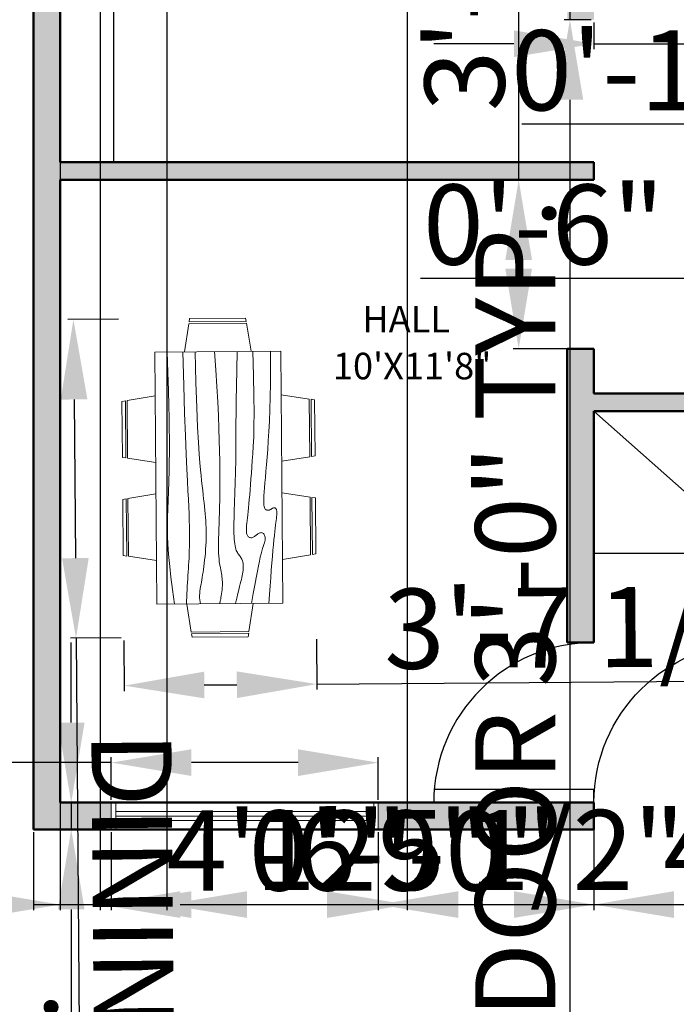
# Model space of a CAD drawing. Units: inches. Extents: x -261 to 409, y 193 to 762.
# Tile 3 of 6: x -35 to 113, y 384 to 605. Entities that reach past the tile are written whole.
import ezdxf

# ---------------------------------------------------------------- set-up
doc = ezdxf.new("R2010")
doc.units = ezdxf.units.IN
for name, color, linetype, lineweight in [('A-ANNO-DIMS', 2, 'Continuous', 18), ('A-AREA-IDEN', 7, 'Continuous', 25), ('A-DOOR', 3, 'Continuous', 25), ('A-FLOR-CASE', 9, 'Continuous', 25), ('A-FLOR-STRS', 7, 'Continuous', 25), ('A-FURN', 8, 'Continuous', 18), ('A-GLAZ', 4, 'Continuous', 18), ('A-WALL', 7, 'Continuous', 50), ('A-WALL-PATT', 8, 'Continuous', 13)]:
    doc.layers.add(name, color=color, linetype=linetype, lineweight=lineweight)
doc.styles.get("Standard").update_dxf_attribs({"font": 'arial.ttf'})
doc.dimstyles.new('ISO-25', dxfattribs={"dimtxt": 18, "dimasz": 18, "dimexe": 1.25, "dimexo": 0.625, "dimtad": 1, "dimdec": 1, "dimlunit": 3, "dimtxsty": 'Standard', "dimcen": 2.5, "dimadec": 0, "dimazin": 0, "dimtfac": 1, "dimtdec": 1, "dimtmove": 0, "dimatfit": 3, "dimfxl": 1, "dimarcsym": 0})

# ---------------------------------------------------------------- blocks, each defined once
blk = doc.blocks.new('Dining Set - 36 x 72 in.')
for p, q in [((-22.2343, 26.00059), (-23.4847, 17.99762)), ((-22.2304, 26), (-5.7608, 26)), ((-22, 27.5), (-22.1562, 26.50042)), ((-5.8416, 26.5), (-22.1534, 26.5)), ((-22, 27.5), (-6, 27.5)), ((-5.8437, 26.49966), (-6, 27.5)), ((-4.5152, 17.99762), (-5.7655, 25.99926)), ((5.7657, 26.00059), (4.5153, 17.99762)), ((5.7696, 26), (22.2392, 26)), ((6, 27.5), (5.8438, 26.50042)), ((22.1584, 26.5), (5.8466, 26.5)), ((6, 27.5), (22, 27.5)), ((22.1563, 26.49966), (22, 27.5)), ((23.4848, 17.99762), (22.2345, 25.99926)), ((36, 18), (-36, 18)), ((-36, 18), (-36, -18)), ((36, -18), (36, 18)), ((-44.0006, 8.23428), (-35.9976, 9.48474)), ((44.0006, 8.23428), (35.9976, 9.48474)), ((-45.5, 8), (-44.5004, 8.15617)), ((-45.5, 8), (-45.5, -8)), ((-44.5, -8.15843), (-44.5, 8.15338)), ((-44, 8.23041), (-44, -8.23915)), ((44, 8.23041), (44, -8.23915)), ((44.5, -8.15843), (44.5, 8.15338)), ((45.5, 8), (44.5005, 8.15617)), ((45.5, 8), (45.5, -8)), ((-44.4997, -8.15631), (-45.5, -8)), ((-35.9976, -9.48476), (-43.9993, -8.2345)), ((35.9976, -9.48476), (43.9993, -8.2345)), ((44.4997, -8.15631), (45.5, -8)), ((-36, -18), (36, -18)), ((-22.2343, -26.0006), (-23.4847, -17.99762)), ((-4.5152, -17.99762), (-5.7655, -25.99928)), ((5.7657, -26.0006), (4.5153, -17.99762)), ((23.4848, -17.99762), (22.2345, -25.99928)), ((-22.2304, -26), (-5.7608, -26)), ((-22, -27.5), (-22.1562, -26.50044)), ((-5.8416, -26.5), (-22.1534, -26.5)), ((-22, -27.5), (-6, -27.5)), ((-5.8437, -26.49967), (-6, -27.5)), ((5.7696, -26), (22.2392, -26)), ((6, -27.5), (5.8438, -26.50044)), ((22.1584, -26.5), (5.8466, -26.5)), ((6, -27.5), (22, -27.5)), ((22.1563, -26.49967), (22, -27.5))]:
    blk.add_line(p, q)
for points in [[(-36, 15), (-31.1772, 14.97754), (-26.8079, 14.91406), (-22.8538, 14.81543), (-19.276, 14.6875), (-16.0362, 14.53613), (-13.0957, 14.36718), (-10.4159, 14.18652), (-7.9583, 14), (-5.6904, 13.81315), (-3.6035, 13.63021), (-1.6954, 13.45508), (0.0365, 13.29166), (1.5945, 13.14388), (2.9811, 13.01562), (4.1988, 12.9108), (5.25, 12.83333), (6.1393, 12.78613), (6.8802, 12.76823), (7.4883, 12.77767), (7.9792, 12.8125), (8.3685, 12.87077), (8.6719, 12.95052), (8.9049, 13.0498), (9.0833, 13.16666), (9.2205, 13.29899), (9.3216, 13.44401), (9.3895, 13.59879), (9.4271, 13.76041), (9.4373, 13.92594), (9.4232, 14.09245), (9.3875, 14.257), (9.3333, 14.41666), (9.2638, 14.56917), (9.1836, 14.71484), (9.0975, 14.85465), (9.0104, 14.98958), (8.9272, 15.1206), (8.8529, 15.2487), (8.7922, 15.37483), (8.75, 15.5), (8.7305, 15.62467), (8.7344, 15.74739), (8.7617, 15.86621), (8.8125, 15.97916), (8.8867, 16.08431), (8.9844, 16.17968), (9.1055, 16.26334), (9.25, 16.33333), (9.4189, 16.38802), (9.6172, 16.42708), (9.8506, 16.45052), (10.125, 16.45833), (10.4463, 16.45052), (10.8203, 16.42708), (11.2529, 16.38802), (11.75, 16.33333), (12.3184, 16.26318), (12.9694, 16.17838), (13.7151, 16.07991), (14.5677, 15.96875), (15.5395, 15.84586), (16.6426, 15.71224), (17.8893, 15.56884), (19.2917, 15.41666), (20.859, 15.25667), (22.5879, 15.08984), (24.4721, 14.91715), (26.5052, 14.73958), (28.6809, 14.5581), (30.9929, 14.3737), (33.4347, 14.18733), (36, 14)], [(-36, 10), (-28.9766, 10.14274), (-23.1725, 10.20442), (-18.4241, 10.19775), (-14.5677, 10.13541), (-11.4399, 10.03011), (-8.877, 9.89453), (-6.7154, 9.74137), (-4.7917, 9.58333), (-2.9698, 9.43082), (-1.2246, 9.28515), (0.4415, 9.14534), (2.026, 9.01041), (3.5266, 8.87939), (4.9408, 8.7513), (6.266, 8.62516), (7.5, 8.5), (8.6411, 8.37549), (9.6914, 8.2539), (10.6538, 8.13818), (11.5312, 8.03125), (12.3267, 7.93603), (13.043, 7.85547), (13.6831, 7.79248), (14.25, 7.75), (14.7471, 7.7303), (15.1797, 7.73307), (15.5537, 7.75732), (15.875, 7.80208), (16.1494, 7.86637), (16.3828, 7.94922), (16.5811, 8.04964), (16.75, 8.16666), (16.8944, 8.29915), (17.0143, 8.44531), (17.1089, 8.60319), (17.1771, 8.77083), (17.218, 8.94629), (17.2305, 9.1276), (17.2137, 9.31282), (17.1667, 9.5), (17.0895, 9.6875), (16.987, 9.875), (16.8649, 10.0625), (16.7292, 10.25), (16.5856, 10.4375), (16.4401, 10.625), (16.2985, 10.8125), (16.1667, 11), (16.05, 11.18733), (15.9518, 11.3737), (15.8752, 11.5581), (15.8229, 11.73958), (15.798, 11.91715), (15.8034, 12.08984), (15.842, 12.25667), (15.9167, 12.41666), (16.0295, 12.56836), (16.1784, 12.70833), (16.3605, 12.83268), (16.5729, 12.9375), (16.8127, 13.01888), (17.0768, 13.07291), (17.3625, 13.0957), (17.6667, 13.08333), (17.9894, 13.03312), (18.3418, 12.94726), (18.7382, 12.82918), (19.1927, 12.68229), (19.7195, 12.51001), (20.3327, 12.31575), (21.0465, 12.10294), (21.875, 11.875), (22.8357, 11.63354), (23.959, 11.37304), (25.2786, 11.08618), (26.8282, 10.76562), (28.6414, 10.40405), (30.752, 9.99414), (33.1936, 9.52856), (36, 9)], [(-36, 5.5), (-30.7157, 5.3348), (-26.069, 5.20963), (-21.9946, 5.11767), (-18.4271, 5.05208), (-15.3009, 5.00602), (-12.5508, 4.97265), (-10.1112, 4.94515), (-7.9167, 4.91666), (-5.909, 4.88167), (-4.0586, 4.83984), (-2.3429, 4.79215), (-0.7396, 4.73958), (0.7739, 4.6831), (2.22, 4.6237), (3.6213, 4.56233), (5, 4.5), (6.373, 4.43782), (7.7344, 4.3776), (9.0723, 4.32129), (10.375, 4.27083), (11.6309, 4.22819), (12.8281, 4.19531), (13.9551, 4.17415), (15, 4.16666), (15.954, 4.17448), (16.819, 4.19791), (17.6001, 4.23698), (18.3021, 4.29166), (18.9299, 4.36198), (19.4883, 4.44791), (19.9823, 4.54948), (20.4167, 4.66666), (20.7969, 4.79899), (21.1302, 4.94401), (21.4245, 5.09879), (21.6875, 5.26041), (21.9271, 5.42594), (22.1511, 5.59245), (22.3672, 5.757), (22.5834, 5.91666), (22.8065, 6.06868), (23.0404, 6.21093), (23.2879, 6.34147), (23.5521, 6.45833), (23.8358, 6.55957), (24.142, 6.64323), (24.4735, 6.70735), (24.8334, 6.75), (25.2235, 6.76969), (25.642, 6.76692), (26.0858, 6.74267), (26.5521, 6.69791), (27.0379, 6.63362), (27.5404, 6.55078), (28.0565, 6.45036), (28.5834, 6.33333), (29.1242, 6.19987), (29.7071, 6.04687), (30.3661, 5.87044), (31.1354, 5.66666), (32.0493, 5.43164), (33.142, 5.16146), (34.4475, 4.85221), (36, 4.5)], [(-36, -1), (-30.7915, -0.6591), (-26.0195, -0.38216), (-21.6519, -0.16284), (-17.6563, 0.00521), (-14.0005, 0.12833), (-10.6523, 0.21289), (-7.5796, 0.26522), (-4.75, 0.29166), (-2.134, 0.29793), (0.2878, 0.28711), (2.5317, 0.26163), (4.6146, 0.22396), (6.5529, 0.17651), (8.3633, 0.12174), (10.0623, 0.06209), (11.6667, 0), (13.1899, -0.06201), (14.6341, -0.1211), (15.9982, -0.17432), (17.2813, -0.21875), (18.4823, -0.25147), (19.6003, -0.26953), (20.6343, -0.27002), (21.5834, -0.25), (22.4481, -0.20768), (23.2357, -0.14584), (23.9549, -0.06836), (24.6146, 0.02083), (25.2235, 0.11784), (25.7904, 0.21875), (26.3241, 0.31966), (26.8334, 0.41666), (27.3265, 0.50618), (27.8099, 0.58593), (28.2894, 0.65397), (28.7709, 0.70833), (29.2601, 0.74707), (29.763, 0.76823), (30.2855, 0.76985), (30.8334, 0.75), (31.4088, 0.70784), (31.9994, 0.64713), (32.589, 0.57275), (33.1615, 0.48958), (33.7008, 0.4025), (34.1908, 0.3164), (34.6153, 0.23616), (34.9584, 0.16666), (35.2099, 0.11165), (35.3848, 0.07031), (35.504, 0.04069), (35.5886, 0.02083), (35.6594, 0.00879), (35.7377, 0.0026), (35.8442, 0.00032), (36, 0)], [(-36, -6.5), (-27.1843, -6.31267), (-20.084, -6.1263), (-14.469, -5.9419), (-10.1094, -5.76042), (-6.7752, -5.58285), (-4.2363, -5.41016), (-2.2629, -5.24333), (-0.625, -5.08334), (0.8708, -4.93099), (2.2715, -4.78646), (3.5872, -4.64974), (4.8281, -4.52084), (6.0046, -4.39974), (7.127, -4.28646), (8.2053, -4.18099), (9.25, -4.08334), (10.2705, -3.99382), (11.2734, -3.91407), (12.2647, -3.84603), (13.25, -3.79167), (14.2354, -3.75293), (15.2266, -3.73177), (16.2295, -3.73015), (17.25, -3.75), (18.2912, -3.79248), (19.3451, -3.85547), (20.4009, -3.93604), (21.4479, -4.03125), (22.4754, -4.13819), (23.4727, -4.25391), (24.4289, -4.37549), (25.3334, -4.5), (26.1785, -4.62492), (26.9694, -4.74935), (27.7145, -4.87281), (28.4219, -4.99479), (29.1, -5.11483), (29.7572, -5.23242), (30.4016, -5.34709), (31.0417, -5.45834), (31.6837, -5.56437), (32.3262, -5.65821), (32.9658, -5.73153), (33.599, -5.77604), (34.2224, -5.78345), (34.8327, -5.74545), (35.4264, -5.65373), (36, -5.5)], [(-36, -10), (-26.4022, -9.81299), (-18.4675, -9.62891), (-11.9839, -9.45069), (-6.7396, -9.28125), (-2.5226, -9.12354), (0.8789, -8.98047), (3.6769, -8.85498), (6.0833, -8.75), (8.2767, -8.66765), (10.3021, -8.60677), (12.1712, -8.56543), (13.8958, -8.54167), (15.4876, -8.53353), (16.9583, -8.53907), (18.3197, -8.55632), (19.5834, -8.58334), (20.7616, -8.61841), (21.8685, -8.66081), (22.9188, -8.71004), (23.9271, -8.76563), (24.9081, -8.82707), (25.8763, -8.89388), (26.8465, -8.96558), (27.8334, -9.04167), (28.8474, -9.12118), (29.8828, -9.20117), (30.93, -9.27824), (31.9792, -9.34896), (33.0205, -9.40991), (34.0443, -9.45768), (35.0407, -9.48885), (36, -9.5)], [(-36, -14.5), (-30.0881, -14.33513), (-25.0332, -14.21224), (-20.7312, -14.12647), (-17.0781, -14.07292), (-13.97, -14.04671), (-11.3027, -14.04297), (-8.9724, -14.05681), (-6.875, -14.08334), (-4.9224, -14.11833), (-3.0905, -14.16016), (-1.3709, -14.20785), (0.2448, -14.26042), (1.7647, -14.3169), (3.1973, -14.3763), (4.5507, -14.43767), (5.8333, -14.5), (7.0554, -14.5621), (8.235, -14.62175), (9.3922, -14.67652), (10.5469, -14.72396), (11.7192, -14.76164), (12.929, -14.78711), (14.1965, -14.79794), (15.5417, -14.79167), (16.9933, -14.76424), (18.6152, -14.70508), (20.4804, -14.60197), (22.6615, -14.44271), (25.2312, -14.21509), (28.2624, -13.9069), (31.8277, -13.50594), (36, -13)]]:
    blk.add_lwpolyline(points)
blk = doc.blocks.new('DOOR-SWING-36IN')
for p, q in [((0, 3), (36, 3)), ((36, 0), (36, 3)), ((0, 0), (36, 0))]:
    blk.add_line(p, q)
blk.add_arc((36, 0), 36, 90, 180)
blk = doc.blocks.new('WIN-60IN')
for p, q in [((60, 6), (0, 6)), ((0, 6), (0, 0)), ((1, 6), (1, 0)), ((59, 0), (59, 6)), ((60, 0), (60, 6)), ((59, 4), (1, 4)), ((59, 3), (1, 3)), ((0, 0), (60, 0)), ((59, 2), (1, 2))]:
    blk.add_line(p, q)
blk = doc.blocks.new('*D11')
at = {"layer": 'A-ANNO-DIMS', "color": 0, "lineweight": -2, "transparency": 16777216}
for p, q in [((88.9, 659.26), (88.9, 677.26)), ((93.68, 641.26), (87.65, 641.26)), ((88.9, 641.26), (88.9, 605.26)), ((93.68, 605.26), (87.65, 605.26)), ((88.9, 587.26), (88.9, 376.77))]:
    blk.add_line(p, q, dxfattribs=at)
at = {"layer": 'A-ANNO-DIMS', "color": 0, "transparency": 16777216}
for points in [[(85.9, 659.26), (91.9, 659.26), (88.9, 641.26)], [(85.9, 587.26), (91.9, 587.26), (88.9, 605.26)]]:
    blk.add_solid(points, dxfattribs=at)
at = {"layer": 'Defpoints', "color": 0, "transparency": 16777216}
for p in [(94.3, 641.26), (88.9, 605.26), (94.3, 605.26)]:
    blk.add_point(p, dxfattribs=at)
at = {"layer": 'A-ANNO-DIMS', "color": 0, "transparency": 16777216, "insert": (78.96, 473.02), "char_height": 18, "attachment_point": 5, "rotation": 90}
blk.add_mtext('DOOR 3\'-0" TYP.', dxfattribs=at)
blk = doc.blocks.new('*D12')
at = {"layer": 'A-ANNO-DIMS', "color": 0, "lineweight": -2, "transparency": 16777216}
for p, q in [((94.3, 604.64), (94.3, 598.61)), ((130.3, 604.64), (130.3, 598.61)), ((76.3, 599.86), (58.3, 599.86)), ((94.3, 599.86), (130.3, 599.86)), ((148.3, 599.86), (277.26, 599.86))]:
    blk.add_line(p, q, dxfattribs=at)
at = {"layer": 'A-ANNO-DIMS', "color": 0, "transparency": 16777216}
for points in [[(76.3, 602.86), (76.3, 596.86), (94.3, 599.86)], [(148.3, 602.86), (148.3, 596.86), (130.3, 599.86)]]:
    blk.add_solid(points, dxfattribs=at)
at = {"layer": 'Defpoints', "color": 0, "transparency": 16777216}
for p in [(94.3, 605.26), (130.3, 605.26), (130.3, 599.86)]:
    blk.add_point(p, dxfattribs=at)
at = {"layer": 'A-ANNO-DIMS', "color": 0, "transparency": 16777216, "insert": (221.78, 609.69), "char_height": 18, "attachment_point": 5}
blk.add_mtext('3\'-0" TYP.', dxfattribs=at)
blk = doc.blocks.new('*D15')
at = {"layer": 'A-ANNO-DIMS', "color": 0, "lineweight": -2, "transparency": 16777216}
for p, q in [((-14.2, 438.26), (-261.22, 438.26)), ((-14.2, 429.89), (-14.2, 439.51)), ((27.8, 438.26), (3.8, 438.26)), ((45.8, 429.89), (45.8, 439.51))]:
    blk.add_line(p, q, dxfattribs=at)
at = {"layer": 'A-ANNO-DIMS', "color": 0, "transparency": 16777216}
for points in [[(3.8, 441.26), (3.8, 435.26), (-14.2, 438.26)], [(27.8, 441.26), (27.8, 435.26), (45.8, 438.26)]]:
    blk.add_solid(points, dxfattribs=at)
at = {"layer": 'Defpoints', "color": 0, "transparency": 16777216}
for p in [(-14.2, 438.26), (-14.2, 429.26), (45.8, 429.26)]:
    blk.add_point(p, dxfattribs=at)
at = {"layer": 'A-ANNO-DIMS', "color": 0, "transparency": 16777216, "insert": (-146.71, 448.2), "char_height": 18, "attachment_point": 5}
blk.add_mtext('WINDOW 5\'-0" TYP.', dxfattribs=at)
blk = doc.blocks.new('*D16')
at = {"layer": 'A-ANNO-DIMS', "color": 0, "lineweight": -2, "transparency": 16777216}
for p, q in [((-23.2, 447.26), (-23.2, 465.26)), ((-14.82, 429.26), (-24.45, 429.26)), ((-23.2, 429.26), (-23.2, 423.26)), ((-14.82, 423.26), (-24.45, 423.26)), ((-23.2, 405.26), (-23.2, 276.29))]:
    blk.add_line(p, q, dxfattribs=at)
at = {"layer": 'A-ANNO-DIMS', "color": 0, "transparency": 16777216}
for points in [[(-26.2, 447.26), (-20.2, 447.26), (-23.2, 429.26)], [(-26.2, 405.26), (-20.2, 405.26), (-23.2, 423.26)]]:
    blk.add_solid(points, dxfattribs=at)
at = {"layer": 'Defpoints', "color": 0, "transparency": 16777216}
for p in [(-14.2, 429.26), (-23.2, 423.26), (-14.2, 423.26)]:
    blk.add_point(p, dxfattribs=at)
at = {"layer": 'A-ANNO-DIMS', "color": 0, "transparency": 16777216, "insert": (-33.01, 331.78), "char_height": 18, "attachment_point": 5, "rotation": 90}
blk.add_mtext('0\'-6" TYP.', dxfattribs=at)
blk = doc.blocks.new('*D18')
at = {"layer": 'A-ANNO-DIMS', "color": 0, "lineweight": -2, "transparency": 16777216}
for p, q in [((184.3, 547.06), (55.33, 547.06)), ((202.3, 545.89), (202.3, 548.31)), ((208.3, 547.06), (202.3, 547.06)), ((208.3, 545.89), (208.3, 548.31)), ((226.3, 547.06), (244.3, 547.06))]:
    blk.add_line(p, q, dxfattribs=at)
at = {"layer": 'A-ANNO-DIMS', "color": 0, "transparency": 16777216}
for points in [[(184.3, 550.06), (184.3, 544.06), (202.3, 547.06)], [(226.3, 550.06), (226.3, 544.06), (208.3, 547.06)]]:
    blk.add_solid(points, dxfattribs=at)
at = {"layer": 'Defpoints', "color": 0, "transparency": 16777216}
for p in [(202.3, 547.06), (202.3, 545.26), (208.3, 545.26)]:
    blk.add_point(p, dxfattribs=at)
at = {"layer": 'A-ANNO-DIMS', "color": 0, "transparency": 16777216, "insert": (110.82, 556.88), "char_height": 18, "attachment_point": 5}
blk.add_mtext('0\'-6" TYP.', dxfattribs=at)
blk = doc.blocks.new('*D21')
at = {"layer": 'A-ANNO-DIMS', "color": 0, "lineweight": -2, "transparency": 16777216}
for p, q in [((-12.58, 537.97), (-23.96, 537.88)), ((-22.56, 519.89), (-22.27, 484.23)), ((-12, 466.31), (-23.38, 466.22)), ((-22.13, 466.23), (-19.92, 193.22))]:
    blk.add_line(p, q, dxfattribs=at)
at = {"layer": 'A-ANNO-DIMS', "color": 0, "transparency": 16777216}
for points in [[(-19.56, 519.92), (-25.56, 519.87), (-22.71, 537.89)], [(-19.27, 484.25), (-25.27, 484.2), (-22.13, 466.23)]]:
    blk.add_solid(points, dxfattribs=at)
at = {"layer": 'Defpoints', "color": 0, "transparency": 16777216}
for p in [(-11.96, 537.98), (-22.13, 466.23), (-11.38, 466.31)]:
    blk.add_point(p, dxfattribs=at)
at = {"layer": 'A-ANNO-DIMS', "color": 0, "transparency": 16777216, "insert": (-11.02, 320.8), "char_height": 18, "attachment_point": 5, "rotation": 270.4625}
blk.add_mtext('DINING SET 5\'-11 1/2"', dxfattribs=at)
blk = doc.blocks.new('*D22')
at = {"layer": 'A-ANNO-DIMS', "color": 0, "lineweight": -2, "transparency": 16777216}
for p, q in [((-11.37, 465.69), (-11.28, 454.31)), ((31.94, 466.04), (32.03, 454.66)), ((32.02, 455.91), (141.05, 456.79)), ((6.71, 455.71), (14.02, 455.77))]:
    blk.add_line(p, q, dxfattribs=at)
at = {"layer": 'A-ANNO-DIMS', "color": 0, "transparency": 16777216}
for points in [[(6.68, 458.71), (6.73, 452.71), (-11.29, 455.56)], [(14, 458.77), (14.05, 452.77), (32.02, 455.91)]]:
    blk.add_solid(points, dxfattribs=at)
at = {"layer": 'Defpoints', "color": 0, "transparency": 16777216}
for p in [(-11.38, 466.31), (31.94, 466.66), (32.02, 455.91)]:
    blk.add_point(p, dxfattribs=at)
at = {"layer": 'A-ANNO-DIMS', "color": 0, "transparency": 16777216, "insert": (95.45, 466.36), "char_height": 18, "attachment_point": 5, "rotation": 0.4625}
blk.add_mtext('3\'-7 1/2"', dxfattribs=at)
blk = doc.blocks.new('*D24')
at = {"layer": 'A-ANNO-DIMS', "color": 0, "lineweight": -2, "transparency": 16777216}
for p, q in [((177.2, 579.75), (177.2, 583.01)), ((188.32, 579.75), (188.32, 583.01)), ((159.2, 581.76), (78.11, 581.76)), ((188.32, 581.76), (177.2, 581.76)), ((206.32, 581.76), (224.32, 581.76))]:
    blk.add_line(p, q, dxfattribs=at)
at = {"layer": 'A-ANNO-DIMS', "color": 0, "transparency": 16777216}
for points in [[(159.2, 584.76), (159.2, 578.76), (177.2, 581.76)], [(206.32, 584.76), (206.32, 578.76), (188.32, 581.76)]]:
    blk.add_solid(points, dxfattribs=at)
at = {"layer": 'Defpoints', "color": 0, "transparency": 16777216}
for p in [(177.2, 581.76), (177.2, 579.13), (188.32, 579.13)]:
    blk.add_point(p, dxfattribs=at)
at = {"layer": 'A-ANNO-DIMS', "color": 0, "transparency": 16777216, "insert": (109.65, 591.57), "char_height": 18, "attachment_point": 5}
blk.add_mtext('0\'-11"', dxfattribs=at)
blk = doc.blocks.new('*D27')
at = {"layer": 'A-ANNO-DIMS', "color": 0, "lineweight": -2, "transparency": 16777216}
for p, q in [((-31.7, 422.64), (-31.7, 405.1)), ((-14.2, 422.64), (-14.2, 405.1)), ((-49.7, 406.35), (-67.7, 406.35)), ((-31.7, 406.35), (-14.2, 406.35)), ((3.8, 406.35), (111.15, 406.35))]:
    blk.add_line(p, q, dxfattribs=at)
at = {"layer": 'A-ANNO-DIMS', "color": 0, "transparency": 16777216}
for points in [[(-49.7, 409.35), (-49.7, 403.35), (-31.7, 406.35)], [(3.8, 409.35), (3.8, 403.35), (-14.2, 406.35)]]:
    blk.add_solid(points, dxfattribs=at)
at = {"layer": 'Defpoints', "color": 0, "transparency": 16777216}
for p in [(-31.7, 423.26), (-14.2, 423.26), (-14.2, 406.35)]:
    blk.add_point(p, dxfattribs=at)
at = {"layer": 'A-ANNO-DIMS', "color": 0, "transparency": 16777216, "insert": (66.48, 416.28), "char_height": 18, "attachment_point": 5}
blk.add_mtext('1\'-5 1/2"', dxfattribs=at)
blk = doc.blocks.new('*D28')
at = {"layer": 'A-ANNO-DIMS', "color": 0, "lineweight": -2, "transparency": 16777216}
for p, q in [((45.8, 422.64), (45.8, 405.1)), ((94.3, 422.64), (94.3, 405.1)), ((63.8, 406.35), (76.3, 406.35)), ((94.3, 406.35), (204.07, 406.35))]:
    blk.add_line(p, q, dxfattribs=at)
at = {"layer": 'A-ANNO-DIMS', "color": 0, "transparency": 16777216}
for points in [[(63.8, 409.35), (63.8, 403.35), (45.8, 406.35)], [(76.3, 409.35), (76.3, 403.35), (94.3, 406.35)]]:
    blk.add_solid(points, dxfattribs=at)
at = {"layer": 'Defpoints', "color": 0, "transparency": 16777216}
for p in [(45.8, 423.26), (94.3, 423.26), (94.3, 406.35)]:
    blk.add_point(p, dxfattribs=at)
at = {"layer": 'A-ANNO-DIMS', "color": 0, "transparency": 16777216, "insert": (158.19, 416.28), "char_height": 18, "attachment_point": 5}
blk.add_mtext('4\'-0 1/2"', dxfattribs=at)
blk = doc.blocks.new('*D31')
at = {"layer": 'A-ANNO-DIMS', "color": 0, "lineweight": -2, "transparency": 16777216}
for p, q in [((-25.7, 674.64), (-25.7, 405.1)), ((-16.7, 674.64), (-16.7, 405.1)), ((-43.7, 406.35), (-61.7, 406.35)), ((-25.7, 406.35), (-16.7, 406.35)), ((1.3, 406.35), (68.4, 406.35))]:
    blk.add_line(p, q, dxfattribs=at)
at = {"layer": 'A-ANNO-DIMS', "color": 0, "transparency": 16777216}
for points in [[(-43.7, 409.35), (-43.7, 403.35), (-25.7, 406.35)], [(1.3, 409.35), (1.3, 403.35), (-16.7, 406.35)]]:
    blk.add_solid(points, dxfattribs=at)
at = {"layer": 'Defpoints', "color": 0, "transparency": 16777216}
for p in [(-25.7, 675.26), (-16.7, 675.26), (-16.7, 406.35)]:
    blk.add_point(p, dxfattribs=at)
at = {"layer": 'A-ANNO-DIMS', "color": 0, "transparency": 16777216, "insert": (43.85, 416.17), "char_height": 18, "attachment_point": 5}
blk.add_mtext('0\'-9"', dxfattribs=at)
blk = doc.blocks.new('*D34')
at = {"layer": 'A-ANNO-DIMS', "color": 0, "lineweight": -2, "transparency": 16777216}
for p, q in [((94.3, 428.64), (94.3, 405.1)), ((202.3, 428.64), (202.3, 405.1)), ((112.3, 406.35), (184.3, 406.35))]:
    blk.add_line(p, q, dxfattribs=at)
at = {"layer": 'A-ANNO-DIMS', "color": 0, "transparency": 16777216}
for points in [[(112.3, 409.35), (112.3, 403.35), (94.3, 406.35)], [(184.3, 409.35), (184.3, 403.35), (202.3, 406.35)]]:
    blk.add_solid(points, dxfattribs=at)
at = {"layer": 'Defpoints', "color": 0, "transparency": 16777216}
for p in [(94.3, 429.26), (202.3, 429.26), (202.3, 406.35)]:
    blk.add_point(p, dxfattribs=at)
at = {"layer": 'A-ANNO-DIMS', "color": 0, "transparency": 16777216, "insert": (148.3, 416.17), "char_height": 18, "attachment_point": 5}
blk.add_mtext('9\'-0"', dxfattribs=at)
blk = doc.blocks.new('*D35')
at = {"layer": 'A-ANNO-DIMS', "color": 0, "lineweight": -2, "transparency": 16777216}
for p, q in [((-48.61, 671.26), (-48.61, 689.26)), ((-2.32, 653.26), (-49.86, 653.26)), ((-48.61, 653.26), (-48.61, 629.26)), ((-2.32, 629.26), (-49.86, 629.26)), ((-48.61, 611.26), (-48.61, 543.86))]:
    blk.add_line(p, q, dxfattribs=at)
at = {"layer": 'A-ANNO-DIMS', "color": 0, "transparency": 16777216}
for points in [[(-51.61, 671.26), (-45.61, 671.26), (-48.61, 653.26)], [(-51.61, 611.26), (-45.61, 611.26), (-48.61, 629.26)]]:
    blk.add_solid(points, dxfattribs=at)
at = {"layer": 'Defpoints', "color": 0, "transparency": 16777216}
for p in [(-1.7, 653.26), (-48.61, 629.26), (-1.7, 629.26)]:
    blk.add_point(p, dxfattribs=at)
at = {"layer": 'A-ANNO-DIMS', "color": 0, "transparency": 16777216, "insert": (-58.42, 568.56), "char_height": 18, "attachment_point": 5, "rotation": 90}
blk.add_mtext('2\'-0"', dxfattribs=at)
blk = doc.blocks.new('*D36')
at = {"layer": 'A-ANNO-DIMS', "color": 0, "lineweight": -2, "transparency": 16777216}
for p, q in [((-25.7, 628.64), (-25.7, 405.1)), ((-1.7, 628.64), (-1.7, 405.1)), ((-43.7, 406.35), (-61.7, 406.35)), ((-25.7, 406.35), (-1.7, 406.35)), ((16.3, 406.35), (83.71, 406.35))]:
    blk.add_line(p, q, dxfattribs=at)
at = {"layer": 'A-ANNO-DIMS', "color": 0, "transparency": 16777216}
for points in [[(-43.7, 409.35), (-43.7, 403.35), (-25.7, 406.35)], [(16.3, 409.35), (16.3, 403.35), (-1.7, 406.35)]]:
    blk.add_solid(points, dxfattribs=at)
at = {"layer": 'Defpoints', "color": 0, "transparency": 16777216}
for p in [(-25.7, 629.26), (-1.7, 629.26), (-1.7, 406.35)]:
    blk.add_point(p, dxfattribs=at)
at = {"layer": 'A-ANNO-DIMS', "color": 0, "transparency": 16777216, "insert": (59.01, 416.17), "char_height": 18, "attachment_point": 5}
blk.add_mtext('2\'-0"', dxfattribs=at)
blk = doc.blocks.new('*D42')
at = {"layer": 'A-ANNO-DIMS', "color": 0, "lineweight": -2, "transparency": 16777216}
for p, q in [((112.3, 740.18), (94.3, 740.18)), ((130.3, 461.89), (130.3, 741.43)), ((130.3, 740.18), (138.3, 740.18)), ((138.3, 461.89), (138.3, 741.43)), ((156.3, 740.18), (223.4, 740.18))]:
    blk.add_line(p, q, dxfattribs=at)
at = {"layer": 'A-ANNO-DIMS', "color": 0, "transparency": 16777216}
for points in [[(112.3, 743.18), (112.3, 737.18), (130.3, 740.18)], [(156.3, 743.18), (156.3, 737.18), (138.3, 740.18)]]:
    blk.add_solid(points, dxfattribs=at)
at = {"layer": 'Defpoints', "color": 0, "transparency": 16777216}
for p in [(138.3, 740.18), (130.3, 461.26), (138.3, 461.26)]:
    blk.add_point(p, dxfattribs=at)
at = {"layer": 'A-ANNO-DIMS', "color": 0, "transparency": 16777216, "insert": (198.85, 749.99), "char_height": 18, "attachment_point": 5}
blk.add_mtext('0\'-8"', dxfattribs=at)
blk = doc.blocks.new('*D43')
at = {"layer": 'A-ANNO-DIMS', "color": 0, "lineweight": -2, "transparency": 16777216}
for p, q in [((77.39, 569.26), (77.39, 636.35)), ((93.68, 569.26), (76.14, 569.26)), ((77.39, 549.26), (77.39, 551.26)), ((93.68, 531.26), (76.14, 531.26))]:
    blk.add_line(p, q, dxfattribs=at)
at = {"layer": 'A-ANNO-DIMS', "color": 0, "transparency": 16777216}
for points in [[(74.39, 551.26), (80.39, 551.26), (77.39, 569.26)], [(74.39, 549.26), (80.39, 549.26), (77.39, 531.26)]]:
    blk.add_solid(points, dxfattribs=at)
at = {"layer": 'Defpoints', "color": 0, "transparency": 16777216}
for p in [(77.39, 569.26), (94.3, 569.26), (94.3, 531.26)]:
    blk.add_point(p, dxfattribs=at)
at = {"layer": 'A-ANNO-DIMS', "color": 0, "transparency": 16777216, "insert": (67.57, 611.81), "char_height": 18, "attachment_point": 5, "rotation": 90}
blk.add_mtext('3\'-2"', dxfattribs=at)
blk = doc.blocks.new('*D45')
at = {"layer": 'A-ANNO-DIMS', "color": 0, "lineweight": -2, "transparency": 16777216}
for p, q in [((-48.61, 693.26), (-48.61, 711.26)), ((-26.32, 675.26), (-49.86, 675.26)), ((-48.61, 675.26), (-48.61, 653.26)), ((-2.32, 653.26), (-49.86, 653.26)), ((-48.61, 635.26), (-48.61, 555.87))]:
    blk.add_line(p, q, dxfattribs=at)
at = {"layer": 'A-ANNO-DIMS', "color": 0, "transparency": 16777216}
for points in [[(-51.61, 693.26), (-45.61, 693.26), (-48.61, 675.26)], [(-51.61, 635.26), (-45.61, 635.26), (-48.61, 653.26)]]:
    blk.add_solid(points, dxfattribs=at)
at = {"layer": 'Defpoints', "color": 0, "transparency": 16777216}
for p in [(-25.7, 675.26), (-48.61, 653.26), (-1.7, 653.26)]:
    blk.add_point(p, dxfattribs=at)
at = {"layer": 'A-ANNO-DIMS', "color": 0, "transparency": 16777216, "insert": (-58.42, 586.57), "char_height": 18, "attachment_point": 5, "rotation": 90}
blk.add_mtext('1\'-10"', dxfattribs=at)
blk = doc.blocks.new('*D46')
at = {"layer": 'A-ANNO-DIMS', "color": 0, "lineweight": -2, "transparency": 16777216}
for p, q in [((-1.7, 652.64), (-1.7, 405.1)), ((52.3, 652.64), (52.3, 405.1)), ((16.3, 406.35), (34.3, 406.35))]:
    blk.add_line(p, q, dxfattribs=at)
at = {"layer": 'A-ANNO-DIMS', "color": 0, "transparency": 16777216}
for points in [[(16.3, 409.35), (16.3, 403.35), (-1.7, 406.35)], [(34.3, 409.35), (34.3, 403.35), (52.3, 406.35)]]:
    blk.add_solid(points, dxfattribs=at)
at = {"layer": 'Defpoints', "color": 0, "transparency": 16777216}
for p in [(-1.7, 653.26), (52.3, 653.26), (52.3, 406.35)]:
    blk.add_point(p, dxfattribs=at)
at = {"layer": 'A-ANNO-DIMS', "color": 0, "transparency": 16777216, "insert": (25.3, 416.17), "char_height": 18, "attachment_point": 5}
blk.add_mtext('4\'-6"', dxfattribs=at)

msp = doc.modelspace()

# ---------------------------------------------------------------- hatches: boundary and pattern name
at = {"layer": 'A-WALL-PATT'}
h = msp.add_hatch(color=256, dxfattribs=at)
h.dxf.hatch_style = 1
h.paths.add_polyline_path([(-25.7, 675.26), (-16.7, 675.26), (-16.7, 681.26), (-31.7, 681.26), (-31.7, 423.26), (-14.2, 423.26), (-14.2, 429.26), (-25.7, 429.26), (-25.7, 569.26), (52.3, 569.26), (88.3, 569.26), (94.3, 569.26), (94.3, 573.26), (52.3, 573.26), (-25.7, 573.26), (-25.7, 575.26)])
h.paths.add_polyline_path([(94.3, 429.26), (58.3, 429.26), (45.8, 429.26), (45.8, 423.26), (94.3, 423.26)])
h.paths.add_polyline_path([(208.3, 533.26), (202.3, 533.26), (202.3, 521.26), (150.3, 521.26), (94.3, 521.26), (94.3, 531.26), (88.3, 531.26), (88.3, 465.26), (94.3, 465.26), (94.3, 517.26), (150.3, 517.26), (202.3, 517.26), (202.3, 429.26), (130.3, 429.26), (130.3, 423.26), (208.3, 423.26)])
h.paths.add_polyline_path([(208.3, 577.26), (202.3, 577.26), (202.3, 561.26), (130.3, 561.26), (130.3, 557.26), (150.3, 557.26), (150.3, 551.26), (154.3, 551.26), (154.3, 557.26), (202.3, 557.26), (202.3, 545.26), (208.3, 545.26)])
h.paths.add_polyline_path([(208.3, 633.26), (202.3, 633.26), (202.3, 609.26), (130.3, 609.26), (130.3, 605.26), (130.3, 591.26), (134.3, 591.26), (134.3, 605.26), (202.3, 605.26), (202.3, 589.26), (208.3, 589.26)])
h.paths.add_polyline_path([(208.3, 723.26), (88.3, 723.26), (88.3, 605.26), (94.3, 605.26), (94.3, 641.26), (94.3, 717.26), (202.3, 717.26), (202.3, 693.26), (208.3, 693.26)])
h.paths.add_polyline_path([(52.3, 681.26), (43.3, 681.26), (43.3, 675.26), (52.3, 675.26), (52.3, 677.26)], flags=17)

# ---------------------------------------------------------------- linework, layer by layer
at = {"layer": 'A-FLOR-CASE'}
for p, q in [((-13.7, 629.26), (-13.7, 579.26)), ((-13.7, 579.26), (-13.7, 575.26)), ((-13.7, 575.26), (-13.7, 573.26))]:
    msp.add_line(p, q, dxfattribs=at)
at = {"layer": 'A-FLOR-STRS'}
for q in [(94.3, 517.26), (94.3, 485.26)]:
    msp.add_line((130.3, 485.26), q, dxfattribs=at)
at = {"layer": 'A-WALL'}
for p, q in [((-31.7, 723.26), (-31.7, 423.26)), ((-25.7, 675.26), (-25.7, 575.26)), ((-25.7, 575.26), (-25.7, 573.26)), ((52.3, 573.26), (-25.7, 573.26)), ((52.3, 573.26), (94.3, 573.26)), ((94.3, 573.26), (94.3, 569.26)), ((-25.7, 569.26), (-25.7, 429.26)), ((52.3, 569.26), (-25.7, 569.26)), ((52.3, 569.26), (88.3, 569.26)), ((88.3, 569.26), (94.3, 569.26)), ((88.3, 531.26), (88.3, 465.26)), ((88.3, 531.26), (94.3, 531.26)), ((94.3, 531.26), (94.3, 521.26)), ((150.3, 521.26), (94.3, 521.26)), ((150.3, 517.26), (94.3, 517.26)), ((94.3, 517.26), (94.3, 465.26)), ((88.3, 465.26), (94.3, 465.26)), ((-25.7, 429.26), (94.3, 429.26)), ((94.3, 429.26), (94.3, 423.26)), ((-31.7, 423.26), (94.3, 423.26))]:
    msp.add_line(p, q, dxfattribs=at)

# ---------------------------------------------------------------- block references
at = {"layer": 'A-DOOR'}
msp.add_blockref('DOOR-SWING-36IN', (58.3, 429.26), dxfattribs=at)
at = {"layer": 'A-DOOR', "extrusion": (0, 0, -1), "zscale": -1, "rotation": 269.9999999999998}
msp.add_blockref('DOOR-SWING-36IN', (-130.3, 465.26), dxfattribs=at)
at = {"layer": 'A-FURN', "xscale": 0.7875556027136793, "yscale": 0.7875556027136793, "zscale": 0.7875556027136793, "rotation": 270.4625034589847}
msp.add_blockref('Dining Set - 36 x 72 in.', (9.99, 502.32), dxfattribs=at)
at = {"layer": 'A-GLAZ', "rotation": 180}
msp.add_blockref('WIN-60IN', (45.8, 429.26), dxfattribs=at)

# ---------------------------------------------------------------- texts
at = {"layer": 'A-AREA-IDEN', "char_height": 5.965, "attachment_point": 1}
for s, insert in [('HALL', (42.23, 540.93)), ('10\'X11\'8"', (35.62, 530.39))]:
    msp.add_mtext_dynamic_manual_height_columns(s, width=143.7583, gutter_width=29.83, heights=[0], dxfattribs=dict(at, insert=insert))

# ---------------------------------------------------------------- dimensions: what is measured, and where the dimension line sits
at = {"layer": 'A-ANNO-DIMS'}
for base, p1, p2, picture, middle in [((138.3, 740.18), (130.3, 461.26), (138.3, 461.26), '*D42', (198.85, 749.99)), ((-16.7, 406.35), (-25.7, 675.26), (-16.7, 675.26), '*D31', (43.85, 416.17)), ((52.3, 406.35), (-1.7, 653.26), (52.3, 653.26), '*D46', (25.3, 416.17)), ((-1.7, 406.35), (-25.7, 629.26), (-1.7, 629.26), '*D36', (59.01, 416.17)), ((-14.2, 406.35), (-31.7, 423.26), (-14.2, 423.26), '*D27', (66.48, 416.28)), ((94.3, 406.35), (45.8, 423.26), (94.3, 423.26), '*D28', (158.19, 416.28)), ((202.3, 406.35), (94.3, 429.26), (202.3, 429.26), '*D34', (148.3, 416.17))]:
    dim = msp.add_linear_dim(base=base, p1=p1, p2=p2, dimstyle='ISO-25', override={"dimdec": 1, "dimlfac": 1, "dimrnd": 0, "dimzin": 1, "dimdsep": 46, "dimlunit": 4, "dimfrac": 2}, dxfattribs=at)
    dim.commit()
    dim.dimension.update_dxf_attribs({"geometry": picture, "text_midpoint": middle})
for base, p1, p2, angle, picture, middle in [((-48.61, 653.26), (-25.7, 675.26), (-1.7, 653.26), 90, '*D45', (-58.42, 586.57)), ((-48.61, 629.26), (-1.7, 653.26), (-1.7, 629.26), 90, '*D35', (-58.42, 568.56)), ((77.39, 569.26), (94.3, 531.26), (94.3, 569.26), 90, '*D43', (67.57, 611.81)), ((177.2, 581.76), (188.32, 579.13), (177.2, 579.13), 180, '*D24', (109.65, 591.57)), ((32.02, 455.91), (-11.38, 466.31), (31.94, 466.66), 0.4625, '*D22', (95.45, 466.36))]:
    dim = msp.add_linear_dim(base=base, p1=p1, p2=p2, angle=angle, dimstyle='ISO-25', override={"dimdec": 1, "dimlfac": 1, "dimrnd": 0, "dimzin": 1, "dimdsep": 46, "dimlunit": 4, "dimfrac": 2}, dxfattribs=at)
    dim.commit()
    dim.dimension.update_dxf_attribs({"geometry": picture, "text_midpoint": middle})
for base, p1, p2, angle, text, picture, middle in [((88.9, 605.26), (94.3, 641.26), (94.3, 605.26), 270, 'DOOR <> TYP.', '*D11', (78.96, 473.02)), ((202.3, 547.06), (208.3, 545.26), (202.3, 545.26), 180, '<> TYP.', '*D18', (110.82, 556.88)), ((-22.13, 466.23), (-11.96, 537.98), (-11.38, 466.31), 270.4625, 'DINING SET <>', '*D21', (-11.02, 320.8)), ((-14.2, 438.26), (45.8, 429.26), (-14.2, 429.26), 180, 'WINDOW <> TYP.', '*D15', (-146.71, 448.2)), ((-23.2, 423.26), (-14.2, 429.26), (-14.2, 423.26), 270, '<> TYP.', '*D16', (-33.01, 331.78))]:
    dim = msp.add_linear_dim(base=base, p1=p1, p2=p2, angle=angle, text=text, dimstyle='ISO-25', override={"dimdec": 1, "dimlfac": 1, "dimrnd": 0, "dimzin": 1, "dimdsep": 46, "dimlunit": 4, "dimfrac": 2}, dxfattribs=at)
    dim.commit()
    dim.dimension.update_dxf_attribs({"geometry": picture, "text_midpoint": middle})
dim = msp.add_linear_dim(base=(130.3, 599.86), p1=(94.3, 605.26), p2=(130.3, 605.26), text='<> TYP.', dimstyle='ISO-25', override={"dimdec": 1, "dimlfac": 1, "dimrnd": 0, "dimzin": 1, "dimdsep": 46, "dimlunit": 4, "dimfrac": 2}, dxfattribs=at)
dim.commit()
dim.dimension.update_dxf_attribs({"geometry": '*D12', "text_midpoint": (221.78, 609.69)})

doc.saveas('drawing.dxf')
